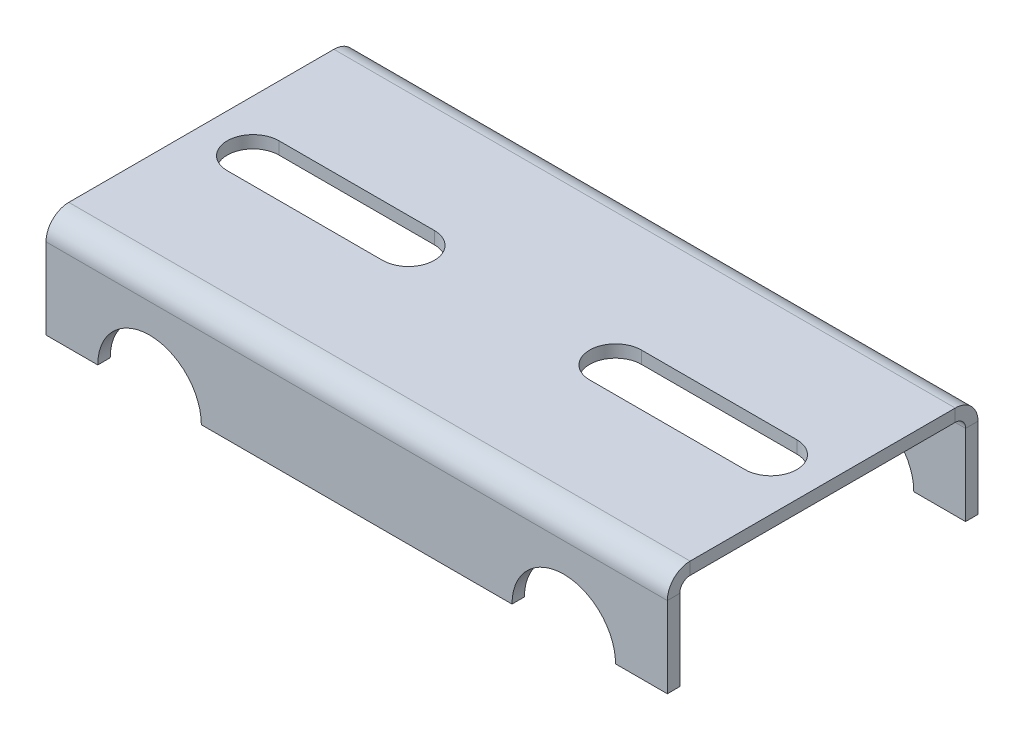
ISO-10303-21;
HEADER;
FILE_DESCRIPTION(('STEP AP214'),'2;1');
FILE_NAME('part.step','',(''),(''),'','','');
FILE_SCHEMA(('AUTOMOTIVE_DESIGN { 1 0 10303 214 1 1 1 1 }'));
ENDSEC;
DATA;
#1=APPLICATION_CONTEXT('core data for automotive mechanical design processes');
#2=APPLICATION_PROTOCOL_DEFINITION('international standard','automotive_design',2000,#1);
#3=PRODUCT_CONTEXT('',#1,'mechanical');
#4=PRODUCT('Part','Part','',(#3));
#5=PRODUCT_RELATED_PRODUCT_CATEGORY('part','',(#4));
#6=PRODUCT_DEFINITION_FORMATION('','',#4);
#7=PRODUCT_DEFINITION_CONTEXT('part definition',#1,'design');
#8=PRODUCT_DEFINITION('design','',#6,#7);
#9=PRODUCT_DEFINITION_SHAPE('','',#8);
#10=(LENGTH_UNIT() NAMED_UNIT(*) SI_UNIT(.MILLI.,.METRE.));
#11=(NAMED_UNIT(*) PLANE_ANGLE_UNIT() SI_UNIT($,.RADIAN.));
#12=(NAMED_UNIT(*) SI_UNIT($,.STERADIAN.) SOLID_ANGLE_UNIT());
#13=UNCERTAINTY_MEASURE_WITH_UNIT(LENGTH_MEASURE(1.E-05),#10,'distance_accuracy_value','');
#14=(GEOMETRIC_REPRESENTATION_CONTEXT(3) GLOBAL_UNCERTAINTY_ASSIGNED_CONTEXT((#13)) GLOBAL_UNIT_ASSIGNED_CONTEXT((#10,
#11,#12)) REPRESENTATION_CONTEXT('',''));
#15=CARTESIAN_POINT('',(0.,0.,0.));
#16=DIRECTION('',(0.,0.,1.));
#17=DIRECTION('',(1.,0.,0.));
#18=AXIS2_PLACEMENT_3D('',#15,#16,#17);
#19=CARTESIAN_POINT('',(0.,-1.524,0.));
#20=DIRECTION('',(0.,-1.,0.));
#21=DIRECTION('',(0.,0.,-1.));
#22=AXIS2_PLACEMENT_3D('',#19,#20,#21);
#23=PLANE('',#22);
#24=CARTESIAN_POINT('',(31.75,-1.524,0.));
#25=DIRECTION('',(0.,1.,0.));
#26=DIRECTION('',(0.,0.,-1.));
#27=AXIS2_PLACEMENT_3D('',#24,#25,#26);
#28=CIRCLE('',#27,3.175);
#29=CARTESIAN_POINT('',(31.75,-1.524,3.175));
#30=VERTEX_POINT('',#29);
#31=CARTESIAN_POINT('',(31.75,-1.524,-3.175));
#32=VERTEX_POINT('',#31);
#33=EDGE_CURVE('E476',#30,#32,#28,.T.);
#34=ORIENTED_EDGE('',*,*,#33,.T.);
#35=DIRECTION('',(-1.,0.,0.));
#36=VECTOR('',#35,1.);
#37=CARTESIAN_POINT('',(31.75,-1.524,-3.175));
#38=LINE('',#37,#36);
#39=CARTESIAN_POINT('',(12.7,-1.524,-3.175));
#40=VERTEX_POINT('',#39);
#41=EDGE_CURVE('E477',#32,#40,#38,.T.);
#42=ORIENTED_EDGE('',*,*,#41,.T.);
#43=CARTESIAN_POINT('',(12.7,-1.524,0.));
#44=DIRECTION('',(0.,1.,0.));
#45=DIRECTION('',(0.,0.,-1.));
#46=AXIS2_PLACEMENT_3D('',#43,#44,#45);
#47=CIRCLE('',#46,3.175);
#48=CARTESIAN_POINT('',(12.7,-1.524,3.175));
#49=VERTEX_POINT('',#48);
#50=EDGE_CURVE('E481',#40,#49,#47,.T.);
#51=ORIENTED_EDGE('',*,*,#50,.T.);
#52=DIRECTION('',(1.,0.,0.));
#53=VECTOR('',#52,1.);
#54=CARTESIAN_POINT('',(31.75,-1.524,3.175));
#55=LINE('',#54,#53);
#56=EDGE_CURVE('E488',#49,#30,#55,.T.);
#57=ORIENTED_EDGE('',*,*,#56,.T.);
#58=EDGE_LOOP('',(#34,#42,#51,#57));
#59=FACE_BOUND('',#58,.T.);
#60=CARTESIAN_POINT('',(-31.75,-1.524,0.));
#61=DIRECTION('',(0.,1.,0.));
#62=DIRECTION('',(0.,0.,1.));
#63=AXIS2_PLACEMENT_3D('',#60,#61,#62);
#64=CIRCLE('',#63,3.175);
#65=CARTESIAN_POINT('',(-31.75,-1.524,-3.175));
#66=VERTEX_POINT('',#65);
#67=CARTESIAN_POINT('',(-31.75,-1.524,3.175));
#68=VERTEX_POINT('',#67);
#69=EDGE_CURVE('E507',#66,#68,#64,.T.);
#70=ORIENTED_EDGE('',*,*,#69,.T.);
#71=DIRECTION('',(1.,0.,0.));
#72=VECTOR('',#71,1.);
#73=CARTESIAN_POINT('',(-31.75,-1.524,3.175));
#74=LINE('',#73,#72);
#75=CARTESIAN_POINT('',(-12.7,-1.524,3.175));
#76=VERTEX_POINT('',#75);
#77=EDGE_CURVE('E512',#68,#76,#74,.T.);
#78=ORIENTED_EDGE('',*,*,#77,.T.);
#79=CARTESIAN_POINT('',(-12.7,-1.524,0.));
#80=DIRECTION('',(0.,1.,0.));
#81=DIRECTION('',(0.,0.,1.));
#82=AXIS2_PLACEMENT_3D('',#79,#80,#81);
#83=CIRCLE('',#82,3.175);
#84=CARTESIAN_POINT('',(-12.7,-1.524,-3.175));
#85=VERTEX_POINT('',#84);
#86=EDGE_CURVE('E513',#76,#85,#83,.T.);
#87=ORIENTED_EDGE('',*,*,#86,.T.);
#88=DIRECTION('',(-1.,0.,0.));
#89=VECTOR('',#88,1.);
#90=CARTESIAN_POINT('',(-31.75,-1.524,-3.175));
#91=LINE('',#90,#89);
#92=EDGE_CURVE('E520',#85,#66,#91,.T.);
#93=ORIENTED_EDGE('',*,*,#92,.T.);
#94=EDGE_LOOP('',(#70,#78,#87,#93));
#95=FACE_BOUND('',#94,.T.);
#96=DIRECTION('',(0.,0.,1.));
#97=VECTOR('',#96,1.);
#98=CARTESIAN_POINT('',(-38.1,-1.524,19.05));
#99=LINE('',#98,#97);
#100=CARTESIAN_POINT('',(-38.1,-1.52400000000001,-16.256));
#101=VERTEX_POINT('',#100);
#102=CARTESIAN_POINT('',(-38.1,-1.524,16.256));
#103=VERTEX_POINT('',#102);
#104=EDGE_CURVE('E13',#101,#103,#99,.T.);
#105=ORIENTED_EDGE('',*,*,#104,.F.);
#106=DIRECTION('',(1.,0.,0.));
#107=VECTOR('',#106,1.);
#108=CARTESIAN_POINT('',(38.1,-1.52400000000001,-16.256));
#109=LINE('',#108,#107);
#110=CARTESIAN_POINT('',(38.1,-1.52400000000001,-16.256));
#111=VERTEX_POINT('',#110);
#112=EDGE_CURVE('E385',#111,#101,#109,.F.);
#113=ORIENTED_EDGE('',*,*,#112,.F.);
#114=DIRECTION('',(0.,0.,-1.));
#115=VECTOR('',#114,1.);
#116=CARTESIAN_POINT('',(38.1,-1.524,19.05));
#117=LINE('',#116,#115);
#118=CARTESIAN_POINT('',(38.1,-1.524,16.256));
#119=VERTEX_POINT('',#118);
#120=EDGE_CURVE('E127',#119,#111,#117,.T.);
#121=ORIENTED_EDGE('',*,*,#120,.F.);
#122=DIRECTION('',(-1.,0.,0.));
#123=VECTOR('',#122,1.);
#124=CARTESIAN_POINT('',(-38.1,-1.524,16.256));
#125=LINE('',#124,#123);
#126=EDGE_CURVE('E466',#103,#119,#125,.F.);
#127=ORIENTED_EDGE('',*,*,#126,.F.);
#128=EDGE_LOOP('',(#105,#113,#121,#127));
#129=FACE_BOUND('',#128,.T.);
#130=ADVANCED_FACE('F122',(#59,#95,#129),#23,.T.);
#131=CARTESIAN_POINT('',(0.,0.,0.));
#132=DIRECTION('',(0.,-1.,0.));
#133=DIRECTION('',(0.,0.,-1.));
#134=AXIS2_PLACEMENT_3D('',#131,#132,#133);
#135=PLANE('',#134);
#136=DIRECTION('',(-1.,0.,0.));
#137=VECTOR('',#136,1.);
#138=CARTESIAN_POINT('',(31.75,0.,-3.175));
#139=LINE('',#138,#137);
#140=CARTESIAN_POINT('',(31.75,0.,-3.175));
#141=VERTEX_POINT('',#140);
#142=CARTESIAN_POINT('',(12.7,0.,-3.175));
#143=VERTEX_POINT('',#142);
#144=EDGE_CURVE('E493',#141,#143,#139,.T.);
#145=ORIENTED_EDGE('',*,*,#144,.F.);
#146=CARTESIAN_POINT('',(31.75,0.,0.));
#147=DIRECTION('',(0.,1.,0.));
#148=DIRECTION('',(0.,0.,-1.));
#149=AXIS2_PLACEMENT_3D('',#146,#147,#148);
#150=CIRCLE('',#149,3.175);
#151=CARTESIAN_POINT('',(31.75,0.,3.175));
#152=VERTEX_POINT('',#151);
#153=EDGE_CURVE('E473',#152,#141,#150,.T.);
#154=ORIENTED_EDGE('',*,*,#153,.F.);
#155=DIRECTION('',(1.,0.,0.));
#156=VECTOR('',#155,1.);
#157=CARTESIAN_POINT('',(31.75,0.,3.175));
#158=LINE('',#157,#156);
#159=CARTESIAN_POINT('',(12.7,0.,3.175));
#160=VERTEX_POINT('',#159);
#161=EDGE_CURVE('E479',#160,#152,#158,.T.);
#162=ORIENTED_EDGE('',*,*,#161,.F.);
#163=CARTESIAN_POINT('',(12.7,0.,0.));
#164=DIRECTION('',(0.,1.,0.));
#165=DIRECTION('',(0.,0.,-1.));
#166=AXIS2_PLACEMENT_3D('',#163,#164,#165);
#167=CIRCLE('',#166,3.175);
#168=EDGE_CURVE('E494',#143,#160,#167,.T.);
#169=ORIENTED_EDGE('',*,*,#168,.F.);
#170=EDGE_LOOP('',(#145,#154,#162,#169));
#171=FACE_BOUND('',#170,.T.);
#172=DIRECTION('',(1.,0.,0.));
#173=VECTOR('',#172,1.);
#174=CARTESIAN_POINT('',(-31.75,0.,3.175));
#175=LINE('',#174,#173);
#176=CARTESIAN_POINT('',(-31.75,0.,3.175));
#177=VERTEX_POINT('',#176);
#178=CARTESIAN_POINT('',(-12.7,0.,3.175));
#179=VERTEX_POINT('',#178);
#180=EDGE_CURVE('E525',#177,#179,#175,.T.);
#181=ORIENTED_EDGE('',*,*,#180,.F.);
#182=CARTESIAN_POINT('',(-31.75,0.,0.));
#183=DIRECTION('',(0.,1.,0.));
#184=DIRECTION('',(0.,0.,1.));
#185=AXIS2_PLACEMENT_3D('',#182,#183,#184);
#186=CIRCLE('',#185,3.175);
#187=CARTESIAN_POINT('',(-31.75,0.,-3.175));
#188=VERTEX_POINT('',#187);
#189=EDGE_CURVE('E501',#188,#177,#186,.T.);
#190=ORIENTED_EDGE('',*,*,#189,.F.);
#191=DIRECTION('',(-1.,0.,0.));
#192=VECTOR('',#191,1.);
#193=CARTESIAN_POINT('',(-31.75,0.,-3.175));
#194=LINE('',#193,#192);
#195=CARTESIAN_POINT('',(-12.7,0.,-3.175));
#196=VERTEX_POINT('',#195);
#197=EDGE_CURVE('E515',#196,#188,#194,.T.);
#198=ORIENTED_EDGE('',*,*,#197,.F.);
#199=CARTESIAN_POINT('',(-12.7,0.,0.));
#200=DIRECTION('',(0.,1.,0.));
#201=DIRECTION('',(0.,0.,1.));
#202=AXIS2_PLACEMENT_3D('',#199,#200,#201);
#203=CIRCLE('',#202,3.175);
#204=EDGE_CURVE('E528',#179,#196,#203,.T.);
#205=ORIENTED_EDGE('',*,*,#204,.F.);
#206=EDGE_LOOP('',(#181,#190,#198,#205));
#207=FACE_BOUND('',#206,.T.);
#208=DIRECTION('',(1.,0.,0.));
#209=VECTOR('',#208,1.);
#210=CARTESIAN_POINT('',(38.1,0.,-16.256));
#211=LINE('',#210,#209);
#212=CARTESIAN_POINT('',(38.1,0.,-16.256));
#213=VERTEX_POINT('',#212);
#214=CARTESIAN_POINT('',(-38.1,0.,-16.256));
#215=VERTEX_POINT('',#214);
#216=EDGE_CURVE('E369',#213,#215,#211,.F.);
#217=ORIENTED_EDGE('',*,*,#216,.T.);
#218=DIRECTION('',(0.,0.,1.));
#219=VECTOR('',#218,1.);
#220=CARTESIAN_POINT('',(-38.1,0.,19.05));
#221=LINE('',#220,#219);
#222=CARTESIAN_POINT('',(-38.1,0.,16.256));
#223=VERTEX_POINT('',#222);
#224=EDGE_CURVE('E123',#215,#223,#221,.T.);
#225=ORIENTED_EDGE('',*,*,#224,.T.);
#226=DIRECTION('',(-1.,0.,0.));
#227=VECTOR('',#226,1.);
#228=CARTESIAN_POINT('',(-38.1,0.,16.256));
#229=LINE('',#228,#227);
#230=CARTESIAN_POINT('',(38.1,0.,16.256));
#231=VERTEX_POINT('',#230);
#232=EDGE_CURVE('E459',#223,#231,#229,.F.);
#233=ORIENTED_EDGE('',*,*,#232,.T.);
#234=DIRECTION('',(0.,0.,-1.));
#235=VECTOR('',#234,1.);
#236=CARTESIAN_POINT('',(38.1,0.,19.05));
#237=LINE('',#236,#235);
#238=EDGE_CURVE('E531',#231,#213,#237,.T.);
#239=ORIENTED_EDGE('',*,*,#238,.T.);
#240=EDGE_LOOP('',(#217,#225,#233,#239));
#241=FACE_BOUND('',#240,.T.);
#242=ADVANCED_FACE('F545',(#171,#207,#241),#135,.F.);
#243=CARTESIAN_POINT('',(38.1,-1.524,19.05));
#244=DIRECTION('',(1.,0.,0.));
#245=DIRECTION('',(0.,0.,-1.));
#246=AXIS2_PLACEMENT_3D('',#243,#244,#245);
#247=PLANE('',#246);
#248=ORIENTED_EDGE('',*,*,#120,.T.);
#249=DIRECTION('',(0.,1.,0.));
#250=VECTOR('',#249,1.);
#251=CARTESIAN_POINT('',(38.1,-1.52400000000001,-16.256));
#252=LINE('',#251,#250);
#253=EDGE_CURVE('E376',#111,#213,#252,.T.);
#254=ORIENTED_EDGE('',*,*,#253,.T.);
#255=ORIENTED_EDGE('',*,*,#238,.F.);
#256=DIRECTION('',(0.,1.,0.));
#257=VECTOR('',#256,1.);
#258=CARTESIAN_POINT('',(38.1,-1.524,16.256));
#259=LINE('',#258,#257);
#260=EDGE_CURVE('E144',#119,#231,#259,.T.);
#261=ORIENTED_EDGE('',*,*,#260,.F.);
#262=EDGE_LOOP('',(#248,#254,#255,#261));
#263=FACE_BOUND('',#262,.T.);
#264=ADVANCED_FACE('F124',(#263),#247,.T.);
#265=CARTESIAN_POINT('',(-38.1,-1.524,19.05));
#266=DIRECTION('',(-1.,0.,0.));
#267=DIRECTION('',(0.,0.,1.));
#268=AXIS2_PLACEMENT_3D('',#265,#266,#267);
#269=PLANE('',#268);
#270=DIRECTION('',(0.,1.,0.));
#271=VECTOR('',#270,1.);
#272=CARTESIAN_POINT('',(-38.1,-1.52400000000001,-16.256));
#273=LINE('',#272,#271);
#274=EDGE_CURVE('E386',#101,#215,#273,.T.);
#275=ORIENTED_EDGE('',*,*,#274,.F.);
#276=ORIENTED_EDGE('',*,*,#104,.T.);
#277=DIRECTION('',(0.,1.,0.));
#278=VECTOR('',#277,1.);
#279=CARTESIAN_POINT('',(-38.1,-1.524,16.256));
#280=LINE('',#279,#278);
#281=EDGE_CURVE('E464',#103,#223,#280,.T.);
#282=ORIENTED_EDGE('',*,*,#281,.T.);
#283=ORIENTED_EDGE('',*,*,#224,.F.);
#284=EDGE_LOOP('',(#275,#276,#282,#283));
#285=FACE_BOUND('',#284,.T.);
#286=ADVANCED_FACE('F548',(#285),#269,.T.);
#287=CARTESIAN_POINT('',(-31.75,-1.524,0.));
#288=DIRECTION('',(0.,1.,0.));
#289=DIRECTION('',(0.,0.,1.));
#290=AXIS2_PLACEMENT_3D('',#287,#288,#289);
#291=CYLINDRICAL_SURFACE('',#290,3.175);
#292=ORIENTED_EDGE('',*,*,#189,.T.);
#293=DIRECTION('',(0.,1.,0.));
#294=VECTOR('',#293,1.);
#295=CARTESIAN_POINT('',(-31.75,-1.524,3.175));
#296=LINE('',#295,#294);
#297=EDGE_CURVE('E524',#68,#177,#296,.T.);
#298=ORIENTED_EDGE('',*,*,#297,.F.);
#299=ORIENTED_EDGE('',*,*,#69,.F.);
#300=DIRECTION('',(0.,1.,0.));
#301=VECTOR('',#300,1.);
#302=CARTESIAN_POINT('',(-31.75,-1.524,-3.175));
#303=LINE('',#302,#301);
#304=EDGE_CURVE('E532',#66,#188,#303,.T.);
#305=ORIENTED_EDGE('',*,*,#304,.T.);
#306=EDGE_LOOP('',(#292,#298,#299,#305));
#307=FACE_BOUND('',#306,.T.);
#308=ADVANCED_FACE('F612',(#307),#291,.F.);
#309=CARTESIAN_POINT('',(-31.75,-1.524,-3.175));
#310=DIRECTION('',(0.,0.,-1.));
#311=DIRECTION('',(-1.,0.,0.));
#312=AXIS2_PLACEMENT_3D('',#309,#310,#311);
#313=PLANE('',#312);
#314=ORIENTED_EDGE('',*,*,#197,.T.);
#315=ORIENTED_EDGE('',*,*,#304,.F.);
#316=ORIENTED_EDGE('',*,*,#92,.F.);
#317=DIRECTION('',(0.,1.,0.));
#318=VECTOR('',#317,1.);
#319=CARTESIAN_POINT('',(-12.7,-1.524,-3.175));
#320=LINE('',#319,#318);
#321=EDGE_CURVE('E534',#85,#196,#320,.T.);
#322=ORIENTED_EDGE('',*,*,#321,.T.);
#323=EDGE_LOOP('',(#314,#315,#316,#322));
#324=FACE_BOUND('',#323,.T.);
#325=ADVANCED_FACE('F625',(#324),#313,.F.);
#326=CARTESIAN_POINT('',(-12.7,-1.524,0.));
#327=DIRECTION('',(0.,1.,0.));
#328=DIRECTION('',(0.,0.,1.));
#329=AXIS2_PLACEMENT_3D('',#326,#327,#328);
#330=CYLINDRICAL_SURFACE('',#329,3.175);
#331=ORIENTED_EDGE('',*,*,#204,.T.);
#332=ORIENTED_EDGE('',*,*,#321,.F.);
#333=ORIENTED_EDGE('',*,*,#86,.F.);
#334=DIRECTION('',(0.,1.,0.));
#335=VECTOR('',#334,1.);
#336=CARTESIAN_POINT('',(-12.7,-1.524,3.175));
#337=LINE('',#336,#335);
#338=EDGE_CURVE('E539',#76,#179,#337,.T.);
#339=ORIENTED_EDGE('',*,*,#338,.T.);
#340=EDGE_LOOP('',(#331,#332,#333,#339));
#341=FACE_BOUND('',#340,.T.);
#342=ADVANCED_FACE('F941',(#341),#330,.F.);
#343=CARTESIAN_POINT('',(-31.75,-1.524,3.175));
#344=DIRECTION('',(0.,0.,1.));
#345=DIRECTION('',(1.,0.,0.));
#346=AXIS2_PLACEMENT_3D('',#343,#344,#345);
#347=PLANE('',#346);
#348=ORIENTED_EDGE('',*,*,#180,.T.);
#349=ORIENTED_EDGE('',*,*,#338,.F.);
#350=ORIENTED_EDGE('',*,*,#77,.F.);
#351=ORIENTED_EDGE('',*,*,#297,.T.);
#352=EDGE_LOOP('',(#348,#349,#350,#351));
#353=FACE_BOUND('',#352,.T.);
#354=ADVANCED_FACE('F932',(#353),#347,.F.);
#355=CARTESIAN_POINT('',(31.75,-1.524,0.));
#356=DIRECTION('',(0.,1.,0.));
#357=DIRECTION('',(0.,0.,1.));
#358=AXIS2_PLACEMENT_3D('',#355,#356,#357);
#359=CYLINDRICAL_SURFACE('',#358,3.175);
#360=ORIENTED_EDGE('',*,*,#153,.T.);
#361=DIRECTION('',(0.,1.,0.));
#362=VECTOR('',#361,1.);
#363=CARTESIAN_POINT('',(31.75,-1.524,-3.175));
#364=LINE('',#363,#362);
#365=EDGE_CURVE('E490',#32,#141,#364,.T.);
#366=ORIENTED_EDGE('',*,*,#365,.F.);
#367=ORIENTED_EDGE('',*,*,#33,.F.);
#368=DIRECTION('',(0.,1.,0.));
#369=VECTOR('',#368,1.);
#370=CARTESIAN_POINT('',(31.75,-1.524,3.175));
#371=LINE('',#370,#369);
#372=EDGE_CURVE('E497',#30,#152,#371,.T.);
#373=ORIENTED_EDGE('',*,*,#372,.T.);
#374=EDGE_LOOP('',(#360,#366,#367,#373));
#375=FACE_BOUND('',#374,.T.);
#376=ADVANCED_FACE('F923',(#375),#359,.F.);
#377=CARTESIAN_POINT('',(31.75,-1.524,3.175));
#378=DIRECTION('',(0.,0.,1.));
#379=DIRECTION('',(1.,0.,0.));
#380=AXIS2_PLACEMENT_3D('',#377,#378,#379);
#381=PLANE('',#380);
#382=ORIENTED_EDGE('',*,*,#161,.T.);
#383=ORIENTED_EDGE('',*,*,#372,.F.);
#384=ORIENTED_EDGE('',*,*,#56,.F.);
#385=DIRECTION('',(0.,1.,0.));
#386=VECTOR('',#385,1.);
#387=CARTESIAN_POINT('',(12.7,-1.524,3.175));
#388=LINE('',#387,#386);
#389=EDGE_CURVE('E505',#49,#160,#388,.T.);
#390=ORIENTED_EDGE('',*,*,#389,.T.);
#391=EDGE_LOOP('',(#382,#383,#384,#390));
#392=FACE_BOUND('',#391,.T.);
#393=ADVANCED_FACE('F918',(#392),#381,.F.);
#394=CARTESIAN_POINT('',(12.7,-1.524,0.));
#395=DIRECTION('',(0.,1.,0.));
#396=DIRECTION('',(0.,0.,1.));
#397=AXIS2_PLACEMENT_3D('',#394,#395,#396);
#398=CYLINDRICAL_SURFACE('',#397,3.175);
#399=ORIENTED_EDGE('',*,*,#168,.T.);
#400=ORIENTED_EDGE('',*,*,#389,.F.);
#401=ORIENTED_EDGE('',*,*,#50,.F.);
#402=DIRECTION('',(0.,1.,0.));
#403=VECTOR('',#402,1.);
#404=CARTESIAN_POINT('',(12.7,-1.524,-3.175));
#405=LINE('',#404,#403);
#406=EDGE_CURVE('E502',#40,#143,#405,.T.);
#407=ORIENTED_EDGE('',*,*,#406,.T.);
#408=EDGE_LOOP('',(#399,#400,#401,#407));
#409=FACE_BOUND('',#408,.T.);
#410=ADVANCED_FACE('F906',(#409),#398,.F.);
#411=CARTESIAN_POINT('',(31.75,-1.524,-3.175));
#412=DIRECTION('',(0.,0.,-1.));
#413=DIRECTION('',(-1.,0.,0.));
#414=AXIS2_PLACEMENT_3D('',#411,#412,#413);
#415=PLANE('',#414);
#416=ORIENTED_EDGE('',*,*,#144,.T.);
#417=ORIENTED_EDGE('',*,*,#406,.F.);
#418=ORIENTED_EDGE('',*,*,#41,.F.);
#419=ORIENTED_EDGE('',*,*,#365,.T.);
#420=EDGE_LOOP('',(#416,#417,#418,#419));
#421=FACE_BOUND('',#420,.T.);
#422=ADVANCED_FACE('F892',(#421),#415,.F.);
#423=CARTESIAN_POINT('',(38.1,-2.794,16.256));
#424=DIRECTION('',(1.,0.,0.));
#425=DIRECTION('',(0.,0.,-1.));
#426=AXIS2_PLACEMENT_3D('',#423,#424,#425);
#427=PLANE('',#426);
#428=DIRECTION('',(0.,0.,1.));
#429=VECTOR('',#428,1.);
#430=CARTESIAN_POINT('',(38.1,-2.794,19.05));
#431=LINE('',#430,#429);
#432=CARTESIAN_POINT('',(38.1,-2.79399999999999,17.526));
#433=VERTEX_POINT('',#432);
#434=CARTESIAN_POINT('',(38.1,-2.79399999999999,19.05));
#435=VERTEX_POINT('',#434);
#436=EDGE_CURVE('E387',#433,#435,#431,.T.);
#437=ORIENTED_EDGE('',*,*,#436,.F.);
#438=CARTESIAN_POINT('',(38.1,-2.794,16.256));
#439=DIRECTION('',(-1.,0.,0.));
#440=DIRECTION('',(0.,0.,1.));
#441=AXIS2_PLACEMENT_3D('',#438,#439,#440);
#442=CIRCLE('',#441,1.27);
#443=EDGE_CURVE('E461',#119,#433,#442,.F.);
#444=ORIENTED_EDGE('',*,*,#443,.F.);
#445=ORIENTED_EDGE('',*,*,#260,.T.);
#446=CARTESIAN_POINT('',(38.1,-2.794,16.256));
#447=DIRECTION('',(-1.,0.,0.));
#448=DIRECTION('',(0.,0.,1.));
#449=AXIS2_PLACEMENT_3D('',#446,#447,#448);
#450=CIRCLE('',#449,2.794);
#451=EDGE_CURVE('E460',#231,#435,#450,.F.);
#452=ORIENTED_EDGE('',*,*,#451,.T.);
#453=EDGE_LOOP('',(#437,#444,#445,#452));
#454=FACE_BOUND('',#453,.T.);
#455=ADVANCED_FACE('F590',(#454),#427,.T.);
#456=CARTESIAN_POINT('',(-38.1,-2.794,16.256));
#457=DIRECTION('',(1.,0.,0.));
#458=DIRECTION('',(0.,0.,-1.));
#459=AXIS2_PLACEMENT_3D('',#456,#457,#458);
#460=PLANE('',#459);
#461=CARTESIAN_POINT('',(-38.1,-2.794,16.256));
#462=DIRECTION('',(-1.,0.,0.));
#463=DIRECTION('',(0.,0.,1.));
#464=AXIS2_PLACEMENT_3D('',#461,#462,#463);
#465=CIRCLE('',#464,1.27);
#466=CARTESIAN_POINT('',(-38.1,-2.79399999999999,17.526));
#467=VERTEX_POINT('',#466);
#468=EDGE_CURVE('E392',#467,#103,#465,.T.);
#469=ORIENTED_EDGE('',*,*,#468,.F.);
#470=DIRECTION('',(0.,0.,1.));
#471=VECTOR('',#470,1.);
#472=CARTESIAN_POINT('',(-38.1,-2.794,17.526));
#473=LINE('',#472,#471);
#474=CARTESIAN_POINT('',(-38.1,-2.794,19.05));
#475=VERTEX_POINT('',#474);
#476=EDGE_CURVE('E446',#467,#475,#473,.T.);
#477=ORIENTED_EDGE('',*,*,#476,.T.);
#478=CARTESIAN_POINT('',(-38.1,-2.794,16.256));
#479=DIRECTION('',(-1.,0.,0.));
#480=DIRECTION('',(0.,0.,1.));
#481=AXIS2_PLACEMENT_3D('',#478,#479,#480);
#482=CIRCLE('',#481,2.794);
#483=EDGE_CURVE('E458',#475,#223,#482,.T.);
#484=ORIENTED_EDGE('',*,*,#483,.T.);
#485=ORIENTED_EDGE('',*,*,#281,.F.);
#486=EDGE_LOOP('',(#469,#477,#484,#485));
#487=FACE_BOUND('',#486,.T.);
#488=ADVANCED_FACE('F552',(#487),#460,.F.);
#489=CARTESIAN_POINT('',(-38.1,-2.794,16.256));
#490=DIRECTION('',(-1.,0.,0.));
#491=DIRECTION('',(0.,0.,1.));
#492=AXIS2_PLACEMENT_3D('',#489,#490,#491);
#493=CYLINDRICAL_SURFACE('',#492,2.794);
#494=ORIENTED_EDGE('',*,*,#232,.F.);
#495=ORIENTED_EDGE('',*,*,#483,.F.);
#496=DIRECTION('',(-1.,0.,0.));
#497=VECTOR('',#496,1.);
#498=CARTESIAN_POINT('',(38.1,-2.794,19.05));
#499=LINE('',#498,#497);
#500=EDGE_CURVE('E450',#475,#435,#499,.F.);
#501=ORIENTED_EDGE('',*,*,#500,.T.);
#502=ORIENTED_EDGE('',*,*,#451,.F.);
#503=EDGE_LOOP('',(#494,#495,#501,#502));
#504=FACE_BOUND('',#503,.T.);
#505=ADVANCED_FACE('F553',(#504),#493,.T.);
#506=CARTESIAN_POINT('',(-38.1,-2.794,16.256));
#507=DIRECTION('',(-1.,0.,0.));
#508=DIRECTION('',(0.,0.,1.));
#509=AXIS2_PLACEMENT_3D('',#506,#507,#508);
#510=CYLINDRICAL_SURFACE('',#509,1.27);
#511=ORIENTED_EDGE('',*,*,#126,.T.);
#512=ORIENTED_EDGE('',*,*,#443,.T.);
#513=DIRECTION('',(-1.,0.,0.));
#514=VECTOR('',#513,1.);
#515=CARTESIAN_POINT('',(38.1,-2.794,17.526));
#516=LINE('',#515,#514);
#517=EDGE_CURVE('E451',#433,#467,#516,.T.);
#518=ORIENTED_EDGE('',*,*,#517,.T.);
#519=ORIENTED_EDGE('',*,*,#468,.T.);
#520=EDGE_LOOP('',(#511,#512,#518,#519));
#521=FACE_BOUND('',#520,.T.);
#522=ADVANCED_FACE('F593',(#521),#510,.F.);
#523=CARTESIAN_POINT('',(-38.1,-1.52399999999999,19.05));
#524=DIRECTION('',(-1.,0.,0.));
#525=DIRECTION('',(0.,-1.,0.));
#526=AXIS2_PLACEMENT_3D('',#523,#524,#525);
#527=PLANE('',#526);
#528=DIRECTION('',(0.,-1.,0.));
#529=VECTOR('',#528,1.);
#530=CARTESIAN_POINT('',(-38.1,-1.52399999999999,19.05));
#531=LINE('',#530,#529);
#532=CARTESIAN_POINT('',(-38.1,-12.7,19.05));
#533=VERTEX_POINT('',#532);
#534=EDGE_CURVE('E406',#533,#475,#531,.F.);
#535=ORIENTED_EDGE('',*,*,#534,.T.);
#536=ORIENTED_EDGE('',*,*,#476,.F.);
#537=DIRECTION('',(0.,1.,0.));
#538=VECTOR('',#537,1.);
#539=CARTESIAN_POINT('',(-38.1,-12.7,17.526));
#540=LINE('',#539,#538);
#541=CARTESIAN_POINT('',(-38.1,-12.7,17.526));
#542=VERTEX_POINT('',#541);
#543=EDGE_CURVE('E430',#542,#467,#540,.T.);
#544=ORIENTED_EDGE('',*,*,#543,.F.);
#545=DIRECTION('',(0.,0.,-1.));
#546=VECTOR('',#545,1.);
#547=CARTESIAN_POINT('',(-38.1,-12.7,19.05));
#548=LINE('',#547,#546);
#549=EDGE_CURVE('E395',#533,#542,#548,.T.);
#550=ORIENTED_EDGE('',*,*,#549,.F.);
#551=EDGE_LOOP('',(#535,#536,#544,#550));
#552=FACE_BOUND('',#551,.T.);
#553=ADVANCED_FACE('F563',(#552),#527,.T.);
#554=CARTESIAN_POINT('',(38.1,-12.7,19.05));
#555=DIRECTION('',(1.,0.,0.));
#556=DIRECTION('',(0.,1.,0.));
#557=AXIS2_PLACEMENT_3D('',#554,#555,#556);
#558=PLANE('',#557);
#559=DIRECTION('',(0.,-1.,0.));
#560=VECTOR('',#559,1.);
#561=CARTESIAN_POINT('',(38.1,-12.6999999999999,17.526));
#562=LINE('',#561,#560);
#563=CARTESIAN_POINT('',(38.1,-12.6999999999998,17.526));
#564=VERTEX_POINT('',#563);
#565=EDGE_CURVE('E444',#433,#564,#562,.T.);
#566=ORIENTED_EDGE('',*,*,#565,.F.);
#567=ORIENTED_EDGE('',*,*,#436,.T.);
#568=DIRECTION('',(0.,1.,0.));
#569=VECTOR('',#568,1.);
#570=CARTESIAN_POINT('',(38.1,-12.7,19.05));
#571=LINE('',#570,#569);
#572=CARTESIAN_POINT('',(38.1,-12.7,19.05));
#573=VERTEX_POINT('',#572);
#574=EDGE_CURVE('E424',#435,#573,#571,.F.);
#575=ORIENTED_EDGE('',*,*,#574,.T.);
#576=DIRECTION('',(0.,0.,-1.));
#577=VECTOR('',#576,1.);
#578=CARTESIAN_POINT('',(38.1,-12.7,19.05));
#579=LINE('',#578,#577);
#580=EDGE_CURVE('E404',#573,#564,#579,.T.);
#581=ORIENTED_EDGE('',*,*,#580,.T.);
#582=EDGE_LOOP('',(#566,#567,#575,#581));
#583=FACE_BOUND('',#582,.T.);
#584=ADVANCED_FACE('F582',(#583),#558,.T.);
#585=CARTESIAN_POINT('',(-25.4,-12.7,19.05));
#586=DIRECTION('',(0.,0.,-1.));
#587=DIRECTION('',(0.,1.,0.));
#588=AXIS2_PLACEMENT_3D('',#585,#586,#587);
#589=PLANE('',#588);
#590=ORIENTED_EDGE('',*,*,#500,.F.);
#591=ORIENTED_EDGE('',*,*,#534,.F.);
#592=DIRECTION('',(1.,0.,0.));
#593=VECTOR('',#592,1.);
#594=CARTESIAN_POINT('',(-38.1,-12.7,19.05));
#595=LINE('',#594,#593);
#596=CARTESIAN_POINT('',(-31.75,-12.7,19.05));
#597=VERTEX_POINT('',#596);
#598=EDGE_CURVE('E407',#597,#533,#595,.F.);
#599=ORIENTED_EDGE('',*,*,#598,.F.);
#600=CARTESIAN_POINT('',(-25.4,-12.7,19.05));
#601=DIRECTION('',(0.,0.,-1.));
#602=DIRECTION('',(0.,1.,0.));
#603=AXIS2_PLACEMENT_3D('',#600,#601,#602);
#604=CIRCLE('',#603,6.35);
#605=CARTESIAN_POINT('',(-19.05,-12.7,19.05));
#606=VERTEX_POINT('',#605);
#607=EDGE_CURVE('E413',#606,#597,#604,.F.);
#608=ORIENTED_EDGE('',*,*,#607,.F.);
#609=DIRECTION('',(1.,0.,0.));
#610=VECTOR('',#609,1.);
#611=CARTESIAN_POINT('',(-19.05,-12.7,19.05));
#612=LINE('',#611,#610);
#613=CARTESIAN_POINT('',(19.05,-12.7,19.05));
#614=VERTEX_POINT('',#613);
#615=EDGE_CURVE('E418',#614,#606,#612,.F.);
#616=ORIENTED_EDGE('',*,*,#615,.F.);
#617=CARTESIAN_POINT('',(25.4,-12.7,19.05));
#618=DIRECTION('',(0.,0.,-1.));
#619=DIRECTION('',(0.,1.,0.));
#620=AXIS2_PLACEMENT_3D('',#617,#618,#619);
#621=CIRCLE('',#620,6.35);
#622=CARTESIAN_POINT('',(31.75,-12.7,19.05));
#623=VERTEX_POINT('',#622);
#624=EDGE_CURVE('E417',#623,#614,#621,.F.);
#625=ORIENTED_EDGE('',*,*,#624,.F.);
#626=DIRECTION('',(1.,0.,0.));
#627=VECTOR('',#626,1.);
#628=CARTESIAN_POINT('',(31.75,-12.7,19.05));
#629=LINE('',#628,#627);
#630=EDGE_CURVE('E422',#573,#623,#629,.F.);
#631=ORIENTED_EDGE('',*,*,#630,.F.);
#632=ORIENTED_EDGE('',*,*,#574,.F.);
#633=EDGE_LOOP('',(#590,#591,#599,#608,#616,#625,#631,#632));
#634=FACE_BOUND('',#633,.T.);
#635=ADVANCED_FACE('F557',(#634),#589,.F.);
#636=CARTESIAN_POINT('',(-25.4,-12.7,17.526));
#637=DIRECTION('',(0.,0.,-1.));
#638=DIRECTION('',(0.,1.,0.));
#639=AXIS2_PLACEMENT_3D('',#636,#637,#638);
#640=PLANE('',#639);
#641=ORIENTED_EDGE('',*,*,#543,.T.);
#642=ORIENTED_EDGE('',*,*,#517,.F.);
#643=ORIENTED_EDGE('',*,*,#565,.T.);
#644=DIRECTION('',(-1.,0.,0.));
#645=VECTOR('',#644,1.);
#646=CARTESIAN_POINT('',(-25.4,-12.7,17.526));
#647=LINE('',#646,#645);
#648=CARTESIAN_POINT('',(31.75,-12.6999999999998,17.526));
#649=VERTEX_POINT('',#648);
#650=EDGE_CURVE('E445',#564,#649,#647,.T.);
#651=ORIENTED_EDGE('',*,*,#650,.T.);
#652=CARTESIAN_POINT('',(25.4,-12.7,17.526));
#653=DIRECTION('',(0.,0.,-1.));
#654=DIRECTION('',(0.,1.,0.));
#655=AXIS2_PLACEMENT_3D('',#652,#653,#654);
#656=CIRCLE('',#655,6.35);
#657=CARTESIAN_POINT('',(19.05,-12.7,17.526));
#658=VERTEX_POINT('',#657);
#659=EDGE_CURVE('E437',#649,#658,#656,.F.);
#660=ORIENTED_EDGE('',*,*,#659,.T.);
#661=DIRECTION('',(-1.,0.,0.));
#662=VECTOR('',#661,1.);
#663=CARTESIAN_POINT('',(-25.4,-12.7,17.526));
#664=LINE('',#663,#662);
#665=CARTESIAN_POINT('',(-19.05,-12.7,17.526));
#666=VERTEX_POINT('',#665);
#667=EDGE_CURVE('E436',#658,#666,#664,.T.);
#668=ORIENTED_EDGE('',*,*,#667,.T.);
#669=CARTESIAN_POINT('',(-25.4,-12.7,17.526));
#670=DIRECTION('',(0.,0.,-1.));
#671=DIRECTION('',(0.,1.,0.));
#672=AXIS2_PLACEMENT_3D('',#669,#670,#671);
#673=CIRCLE('',#672,6.35);
#674=CARTESIAN_POINT('',(-31.75,-12.7,17.526));
#675=VERTEX_POINT('',#674);
#676=EDGE_CURVE('E433',#666,#675,#673,.F.);
#677=ORIENTED_EDGE('',*,*,#676,.T.);
#678=DIRECTION('',(-1.,0.,0.));
#679=VECTOR('',#678,1.);
#680=CARTESIAN_POINT('',(-25.4,-12.7,17.526));
#681=LINE('',#680,#679);
#682=EDGE_CURVE('E427',#675,#542,#681,.T.);
#683=ORIENTED_EDGE('',*,*,#682,.T.);
#684=EDGE_LOOP('',(#641,#642,#643,#651,#660,#668,#677,#683));
#685=FACE_BOUND('',#684,.T.);
#686=ADVANCED_FACE('F592',(#685),#640,.T.);
#687=CARTESIAN_POINT('',(-38.1,-12.7,19.05));
#688=DIRECTION('',(0.,-1.,0.));
#689=DIRECTION('',(0.,0.,-1.));
#690=AXIS2_PLACEMENT_3D('',#687,#688,#689);
#691=PLANE('',#690);
#692=ORIENTED_EDGE('',*,*,#682,.F.);
#693=DIRECTION('',(0.,0.,-1.));
#694=VECTOR('',#693,1.);
#695=CARTESIAN_POINT('',(-31.75,-12.7,19.05));
#696=LINE('',#695,#694);
#697=EDGE_CURVE('E398',#597,#675,#696,.T.);
#698=ORIENTED_EDGE('',*,*,#697,.F.);
#699=ORIENTED_EDGE('',*,*,#598,.T.);
#700=ORIENTED_EDGE('',*,*,#549,.T.);
#701=EDGE_LOOP('',(#692,#698,#699,#700));
#702=FACE_BOUND('',#701,.T.);
#703=ADVANCED_FACE('F566',(#702),#691,.T.);
#704=CARTESIAN_POINT('',(-25.4,-12.7,19.05));
#705=DIRECTION('',(0.,0.,-1.));
#706=DIRECTION('',(0.,1.,0.));
#707=AXIS2_PLACEMENT_3D('',#704,#705,#706);
#708=CYLINDRICAL_SURFACE('',#707,6.35);
#709=ORIENTED_EDGE('',*,*,#676,.F.);
#710=DIRECTION('',(0.,0.,-1.));
#711=VECTOR('',#710,1.);
#712=CARTESIAN_POINT('',(-19.05,-12.7,19.05));
#713=LINE('',#712,#711);
#714=EDGE_CURVE('E397',#606,#666,#713,.T.);
#715=ORIENTED_EDGE('',*,*,#714,.F.);
#716=ORIENTED_EDGE('',*,*,#607,.T.);
#717=ORIENTED_EDGE('',*,*,#697,.T.);
#718=EDGE_LOOP('',(#709,#715,#716,#717));
#719=FACE_BOUND('',#718,.T.);
#720=ADVANCED_FACE('F571',(#719),#708,.F.);
#721=CARTESIAN_POINT('',(-19.05,-12.7,19.05));
#722=DIRECTION('',(0.,-1.,0.));
#723=DIRECTION('',(0.,0.,-1.));
#724=AXIS2_PLACEMENT_3D('',#721,#722,#723);
#725=PLANE('',#724);
#726=ORIENTED_EDGE('',*,*,#667,.F.);
#727=DIRECTION('',(0.,0.,-1.));
#728=VECTOR('',#727,1.);
#729=CARTESIAN_POINT('',(19.05,-12.7,19.05));
#730=LINE('',#729,#728);
#731=EDGE_CURVE('E396',#614,#658,#730,.T.);
#732=ORIENTED_EDGE('',*,*,#731,.F.);
#733=ORIENTED_EDGE('',*,*,#615,.T.);
#734=ORIENTED_EDGE('',*,*,#714,.T.);
#735=EDGE_LOOP('',(#726,#732,#733,#734));
#736=FACE_BOUND('',#735,.T.);
#737=ADVANCED_FACE('F573',(#736),#725,.T.);
#738=CARTESIAN_POINT('',(25.4,-12.7,19.05));
#739=DIRECTION('',(0.,0.,-1.));
#740=DIRECTION('',(0.,1.,0.));
#741=AXIS2_PLACEMENT_3D('',#738,#739,#740);
#742=CYLINDRICAL_SURFACE('',#741,6.35);
#743=ORIENTED_EDGE('',*,*,#659,.F.);
#744=DIRECTION('',(0.,0.,-1.));
#745=VECTOR('',#744,1.);
#746=CARTESIAN_POINT('',(31.75,-12.7,19.05));
#747=LINE('',#746,#745);
#748=EDGE_CURVE('E405',#623,#649,#747,.T.);
#749=ORIENTED_EDGE('',*,*,#748,.F.);
#750=ORIENTED_EDGE('',*,*,#624,.T.);
#751=ORIENTED_EDGE('',*,*,#731,.T.);
#752=EDGE_LOOP('',(#743,#749,#750,#751));
#753=FACE_BOUND('',#752,.T.);
#754=ADVANCED_FACE('F579',(#753),#742,.F.);
#755=CARTESIAN_POINT('',(31.75,-12.7,19.05));
#756=DIRECTION('',(0.,-1.,0.));
#757=DIRECTION('',(1.,0.,0.));
#758=AXIS2_PLACEMENT_3D('',#755,#756,#757);
#759=PLANE('',#758);
#760=ORIENTED_EDGE('',*,*,#650,.F.);
#761=ORIENTED_EDGE('',*,*,#580,.F.);
#762=ORIENTED_EDGE('',*,*,#630,.T.);
#763=ORIENTED_EDGE('',*,*,#748,.T.);
#764=EDGE_LOOP('',(#760,#761,#762,#763));
#765=FACE_BOUND('',#764,.T.);
#766=ADVANCED_FACE('F584',(#765),#759,.T.);
#767=CARTESIAN_POINT('',(-38.1,-2.79400000000001,-16.256));
#768=DIRECTION('',(-1.,0.,0.));
#769=DIRECTION('',(0.,0.,1.));
#770=AXIS2_PLACEMENT_3D('',#767,#768,#769);
#771=PLANE('',#770);
#772=DIRECTION('',(0.,0.,1.));
#773=VECTOR('',#772,1.);
#774=CARTESIAN_POINT('',(-38.1,-2.79399999999999,-19.05));
#775=LINE('',#774,#773);
#776=CARTESIAN_POINT('',(-38.1,-2.794,-17.526));
#777=VERTEX_POINT('',#776);
#778=CARTESIAN_POINT('',(-38.1,-2.794,-19.05));
#779=VERTEX_POINT('',#778);
#780=EDGE_CURVE('E370',#777,#779,#775,.F.);
#781=ORIENTED_EDGE('',*,*,#780,.F.);
#782=CARTESIAN_POINT('',(-38.1,-2.79400000000001,-16.256));
#783=DIRECTION('',(1.,0.,0.));
#784=DIRECTION('',(0.,0.,-1.));
#785=AXIS2_PLACEMENT_3D('',#782,#783,#784);
#786=CIRCLE('',#785,1.27);
#787=EDGE_CURVE('E378',#101,#777,#786,.F.);
#788=ORIENTED_EDGE('',*,*,#787,.F.);
#789=ORIENTED_EDGE('',*,*,#274,.T.);
#790=CARTESIAN_POINT('',(-38.1,-2.79400000000001,-16.256));
#791=DIRECTION('',(1.,0.,0.));
#792=DIRECTION('',(0.,0.,-1.));
#793=AXIS2_PLACEMENT_3D('',#790,#791,#792);
#794=CIRCLE('',#793,2.794);
#795=EDGE_CURVE('E375',#215,#779,#794,.F.);
#796=ORIENTED_EDGE('',*,*,#795,.T.);
#797=EDGE_LOOP('',(#781,#788,#789,#796));
#798=FACE_BOUND('',#797,.T.);
#799=ADVANCED_FACE('F690',(#798),#771,.T.);
#800=CARTESIAN_POINT('',(38.1,-2.79400000000001,-16.256));
#801=DIRECTION('',(-1.,0.,0.));
#802=DIRECTION('',(0.,0.,1.));
#803=AXIS2_PLACEMENT_3D('',#800,#801,#802);
#804=PLANE('',#803);
#805=CARTESIAN_POINT('',(38.1,-2.79400000000001,-16.256));
#806=DIRECTION('',(1.,0.,0.));
#807=DIRECTION('',(0.,0.,-1.));
#808=AXIS2_PLACEMENT_3D('',#805,#806,#807);
#809=CIRCLE('',#808,1.27);
#810=CARTESIAN_POINT('',(38.1,-2.794,-17.526));
#811=VERTEX_POINT('',#810);
#812=EDGE_CURVE('E330',#811,#111,#809,.T.);
#813=ORIENTED_EDGE('',*,*,#812,.F.);
#814=DIRECTION('',(0.,0.,1.));
#815=VECTOR('',#814,1.);
#816=CARTESIAN_POINT('',(38.1,-2.794,-17.526));
#817=LINE('',#816,#815);
#818=CARTESIAN_POINT('',(38.1,-2.79399999999999,-19.05));
#819=VERTEX_POINT('',#818);
#820=EDGE_CURVE('E365',#811,#819,#817,.F.);
#821=ORIENTED_EDGE('',*,*,#820,.T.);
#822=CARTESIAN_POINT('',(38.1,-2.79400000000001,-16.256));
#823=DIRECTION('',(1.,0.,0.));
#824=DIRECTION('',(0.,0.,-1.));
#825=AXIS2_PLACEMENT_3D('',#822,#823,#824);
#826=CIRCLE('',#825,2.794);
#827=EDGE_CURVE('E373',#819,#213,#826,.T.);
#828=ORIENTED_EDGE('',*,*,#827,.T.);
#829=ORIENTED_EDGE('',*,*,#253,.F.);
#830=EDGE_LOOP('',(#813,#821,#828,#829));
#831=FACE_BOUND('',#830,.T.);
#832=ADVANCED_FACE('F629',(#831),#804,.F.);
#833=CARTESIAN_POINT('',(38.1,-2.79400000000001,-16.256));
#834=DIRECTION('',(1.,0.,0.));
#835=DIRECTION('',(0.,0.,-1.));
#836=AXIS2_PLACEMENT_3D('',#833,#834,#835);
#837=CYLINDRICAL_SURFACE('',#836,2.794);
#838=ORIENTED_EDGE('',*,*,#216,.F.);
#839=ORIENTED_EDGE('',*,*,#827,.F.);
#840=DIRECTION('',(1.,0.,0.));
#841=VECTOR('',#840,1.);
#842=CARTESIAN_POINT('',(-38.1,-2.79399999999999,-19.05));
#843=LINE('',#842,#841);
#844=EDGE_CURVE('E317',#819,#779,#843,.F.);
#845=ORIENTED_EDGE('',*,*,#844,.T.);
#846=ORIENTED_EDGE('',*,*,#795,.F.);
#847=EDGE_LOOP('',(#838,#839,#845,#846));
#848=FACE_BOUND('',#847,.T.);
#849=ADVANCED_FACE('F683',(#848),#837,.T.);
#850=CARTESIAN_POINT('',(38.1,-2.79400000000001,-16.256));
#851=DIRECTION('',(1.,0.,0.));
#852=DIRECTION('',(0.,0.,-1.));
#853=AXIS2_PLACEMENT_3D('',#850,#851,#852);
#854=CYLINDRICAL_SURFACE('',#853,1.27);
#855=ORIENTED_EDGE('',*,*,#112,.T.);
#856=ORIENTED_EDGE('',*,*,#787,.T.);
#857=DIRECTION('',(1.,0.,0.));
#858=VECTOR('',#857,1.);
#859=CARTESIAN_POINT('',(-38.1,-2.794,-17.526));
#860=LINE('',#859,#858);
#861=EDGE_CURVE('E362',#777,#811,#860,.T.);
#862=ORIENTED_EDGE('',*,*,#861,.T.);
#863=ORIENTED_EDGE('',*,*,#812,.T.);
#864=EDGE_LOOP('',(#855,#856,#862,#863));
#865=FACE_BOUND('',#864,.T.);
#866=ADVANCED_FACE('F635',(#865),#854,.F.);
#867=CARTESIAN_POINT('',(38.1,-12.7,-19.05));
#868=DIRECTION('',(-1.,0.,0.));
#869=DIRECTION('',(0.,-1.,0.));
#870=AXIS2_PLACEMENT_3D('',#867,#868,#869);
#871=PLANE('',#870);
#872=ORIENTED_EDGE('',*,*,#820,.F.);
#873=DIRECTION('',(0.,1.,0.));
#874=VECTOR('',#873,1.);
#875=CARTESIAN_POINT('',(38.1,-12.7,-17.526));
#876=LINE('',#875,#874);
#877=CARTESIAN_POINT('',(38.1,-12.7,-17.526));
#878=VERTEX_POINT('',#877);
#879=EDGE_CURVE('E322',#811,#878,#876,.F.);
#880=ORIENTED_EDGE('',*,*,#879,.T.);
#881=DIRECTION('',(0.,0.,1.));
#882=VECTOR('',#881,1.);
#883=CARTESIAN_POINT('',(38.1,-12.7,-19.05));
#884=LINE('',#883,#882);
#885=CARTESIAN_POINT('',(38.1,-12.6999999999998,-19.05));
#886=VERTEX_POINT('',#885);
#887=EDGE_CURVE('E321',#886,#878,#884,.T.);
#888=ORIENTED_EDGE('',*,*,#887,.F.);
#889=DIRECTION('',(0.,-1.,0.));
#890=VECTOR('',#889,1.);
#891=CARTESIAN_POINT('',(38.1,-12.6999999999999,-19.05));
#892=LINE('',#891,#890);
#893=EDGE_CURVE('E307',#819,#886,#892,.T.);
#894=ORIENTED_EDGE('',*,*,#893,.F.);
#895=EDGE_LOOP('',(#872,#880,#888,#894));
#896=FACE_BOUND('',#895,.T.);
#897=ADVANCED_FACE('F325',(#896),#871,.F.);
#898=CARTESIAN_POINT('',(-38.1,-1.52399999999999,-19.05));
#899=DIRECTION('',(1.,0.,0.));
#900=DIRECTION('',(0.,1.,0.));
#901=AXIS2_PLACEMENT_3D('',#898,#899,#900);
#902=PLANE('',#901);
#903=ORIENTED_EDGE('',*,*,#780,.T.);
#904=DIRECTION('',(0.,1.,0.));
#905=VECTOR('',#904,1.);
#906=CARTESIAN_POINT('',(-38.1,-12.7,-19.05));
#907=LINE('',#906,#905);
#908=CARTESIAN_POINT('',(-38.1,-12.7,-19.05));
#909=VERTEX_POINT('',#908);
#910=EDGE_CURVE('E342',#909,#779,#907,.T.);
#911=ORIENTED_EDGE('',*,*,#910,.F.);
#912=DIRECTION('',(0.,0.,1.));
#913=VECTOR('',#912,1.);
#914=CARTESIAN_POINT('',(-38.1,-12.7,-19.05));
#915=LINE('',#914,#913);
#916=CARTESIAN_POINT('',(-38.1,-12.7,-17.526));
#917=VERTEX_POINT('',#916);
#918=EDGE_CURVE('E316',#909,#917,#915,.T.);
#919=ORIENTED_EDGE('',*,*,#918,.T.);
#920=DIRECTION('',(0.,-1.,0.));
#921=VECTOR('',#920,1.);
#922=CARTESIAN_POINT('',(-38.1,-1.524,-17.526));
#923=LINE('',#922,#921);
#924=EDGE_CURVE('E356',#917,#777,#923,.F.);
#925=ORIENTED_EDGE('',*,*,#924,.T.);
#926=EDGE_LOOP('',(#903,#911,#919,#925));
#927=FACE_BOUND('',#926,.T.);
#928=ADVANCED_FACE('F642',(#927),#902,.F.);
#929=CARTESIAN_POINT('',(-25.4,-12.7,-19.05));
#930=DIRECTION('',(0.,0.,1.));
#931=DIRECTION('',(0.,1.,0.));
#932=AXIS2_PLACEMENT_3D('',#929,#930,#931);
#933=PLANE('',#932);
#934=ORIENTED_EDGE('',*,*,#844,.F.);
#935=ORIENTED_EDGE('',*,*,#893,.T.);
#936=DIRECTION('',(-1.,0.,0.));
#937=VECTOR('',#936,1.);
#938=CARTESIAN_POINT('',(-25.4,-12.7,-19.05));
#939=LINE('',#938,#937);
#940=CARTESIAN_POINT('',(31.75,-12.6999999999998,-19.05));
#941=VERTEX_POINT('',#940);
#942=EDGE_CURVE('E312',#886,#941,#939,.T.);
#943=ORIENTED_EDGE('',*,*,#942,.T.);
#944=CARTESIAN_POINT('',(25.4,-12.7,-19.05));
#945=DIRECTION('',(0.,0.,1.));
#946=DIRECTION('',(0.,-1.,0.));
#947=AXIS2_PLACEMENT_3D('',#944,#945,#946);
#948=CIRCLE('',#947,6.35);
#949=CARTESIAN_POINT('',(19.05,-12.7,-19.05));
#950=VERTEX_POINT('',#949);
#951=EDGE_CURVE('E335',#941,#950,#948,.T.);
#952=ORIENTED_EDGE('',*,*,#951,.T.);
#953=DIRECTION('',(-1.,0.,0.));
#954=VECTOR('',#953,1.);
#955=CARTESIAN_POINT('',(-25.4,-12.7,-19.05));
#956=LINE('',#955,#954);
#957=CARTESIAN_POINT('',(-19.05,-12.7,-19.05));
#958=VERTEX_POINT('',#957);
#959=EDGE_CURVE('E337',#950,#958,#956,.T.);
#960=ORIENTED_EDGE('',*,*,#959,.T.);
#961=CARTESIAN_POINT('',(-25.4,-12.7,-19.05));
#962=DIRECTION('',(0.,0.,1.));
#963=DIRECTION('',(0.,-1.,0.));
#964=AXIS2_PLACEMENT_3D('',#961,#962,#963);
#965=CIRCLE('',#964,6.35);
#966=CARTESIAN_POINT('',(-31.75,-12.7,-19.05));
#967=VERTEX_POINT('',#966);
#968=EDGE_CURVE('E344',#958,#967,#965,.T.);
#969=ORIENTED_EDGE('',*,*,#968,.T.);
#970=DIRECTION('',(-1.,0.,0.));
#971=VECTOR('',#970,1.);
#972=CARTESIAN_POINT('',(-25.4,-12.7,-19.05));
#973=LINE('',#972,#971);
#974=EDGE_CURVE('E345',#967,#909,#973,.T.);
#975=ORIENTED_EDGE('',*,*,#974,.T.);
#976=ORIENTED_EDGE('',*,*,#910,.T.);
#977=EDGE_LOOP('',(#934,#935,#943,#952,#960,#969,#975,#976));
#978=FACE_BOUND('',#977,.T.);
#979=ADVANCED_FACE('F311',(#978),#933,.F.);
#980=CARTESIAN_POINT('',(-25.4,-12.7,-17.526));
#981=DIRECTION('',(0.,0.,1.));
#982=DIRECTION('',(0.,1.,0.));
#983=AXIS2_PLACEMENT_3D('',#980,#981,#982);
#984=PLANE('',#983);
#985=ORIENTED_EDGE('',*,*,#879,.F.);
#986=ORIENTED_EDGE('',*,*,#861,.F.);
#987=ORIENTED_EDGE('',*,*,#924,.F.);
#988=DIRECTION('',(1.,0.,0.));
#989=VECTOR('',#988,1.);
#990=CARTESIAN_POINT('',(-38.1,-12.7,-17.526));
#991=LINE('',#990,#989);
#992=CARTESIAN_POINT('',(-31.75,-12.7,-17.526));
#993=VERTEX_POINT('',#992);
#994=EDGE_CURVE('E358',#993,#917,#991,.F.);
#995=ORIENTED_EDGE('',*,*,#994,.F.);
#996=CARTESIAN_POINT('',(-25.4,-12.7,-17.526));
#997=DIRECTION('',(0.,0.,1.));
#998=DIRECTION('',(0.,-1.,0.));
#999=AXIS2_PLACEMENT_3D('',#996,#997,#998);
#1000=CIRCLE('',#999,6.35);
#1001=CARTESIAN_POINT('',(-19.05,-12.7,-17.526));
#1002=VERTEX_POINT('',#1001);
#1003=EDGE_CURVE('E352',#1002,#993,#1000,.T.);
#1004=ORIENTED_EDGE('',*,*,#1003,.F.);
#1005=DIRECTION('',(1.,0.,0.));
#1006=VECTOR('',#1005,1.);
#1007=CARTESIAN_POINT('',(-19.05,-12.7,-17.526));
#1008=LINE('',#1007,#1006);
#1009=CARTESIAN_POINT('',(19.05,-12.7,-17.526));
#1010=VERTEX_POINT('',#1009);
#1011=EDGE_CURVE('E355',#1010,#1002,#1008,.F.);
#1012=ORIENTED_EDGE('',*,*,#1011,.F.);
#1013=CARTESIAN_POINT('',(25.4,-12.7,-17.526));
#1014=DIRECTION('',(0.,0.,1.));
#1015=DIRECTION('',(0.,-1.,0.));
#1016=AXIS2_PLACEMENT_3D('',#1013,#1014,#1015);
#1017=CIRCLE('',#1016,6.35);
#1018=CARTESIAN_POINT('',(31.75,-12.7,-17.526));
#1019=VERTEX_POINT('',#1018);
#1020=EDGE_CURVE('E349',#1019,#1010,#1017,.T.);
#1021=ORIENTED_EDGE('',*,*,#1020,.F.);
#1022=DIRECTION('',(1.,0.,0.));
#1023=VECTOR('',#1022,1.);
#1024=CARTESIAN_POINT('',(31.75,-12.7,-17.526));
#1025=LINE('',#1024,#1023);
#1026=EDGE_CURVE('E348',#878,#1019,#1025,.F.);
#1027=ORIENTED_EDGE('',*,*,#1026,.F.);
#1028=EDGE_LOOP('',(#985,#986,#987,#995,#1004,#1012,#1021,#1027));
#1029=FACE_BOUND('',#1028,.T.);
#1030=ADVANCED_FACE('F640',(#1029),#984,.T.);
#1031=CARTESIAN_POINT('',(31.75,-12.7,-19.05));
#1032=DIRECTION('',(0.,1.,0.));
#1033=DIRECTION('',(-1.,0.,0.));
#1034=AXIS2_PLACEMENT_3D('',#1031,#1032,#1033);
#1035=PLANE('',#1034);
#1036=ORIENTED_EDGE('',*,*,#1026,.T.);
#1037=DIRECTION('',(0.,0.,1.));
#1038=VECTOR('',#1037,1.);
#1039=CARTESIAN_POINT('',(31.75,-12.7,-19.05));
#1040=LINE('',#1039,#1038);
#1041=EDGE_CURVE('E328',#941,#1019,#1040,.T.);
#1042=ORIENTED_EDGE('',*,*,#1041,.F.);
#1043=ORIENTED_EDGE('',*,*,#942,.F.);
#1044=ORIENTED_EDGE('',*,*,#887,.T.);
#1045=EDGE_LOOP('',(#1036,#1042,#1043,#1044));
#1046=FACE_BOUND('',#1045,.T.);
#1047=ADVANCED_FACE('F333',(#1046),#1035,.F.);
#1048=CARTESIAN_POINT('',(25.4,-12.7,-19.05));
#1049=DIRECTION('',(0.,0.,1.));
#1050=DIRECTION('',(0.,-1.,0.));
#1051=AXIS2_PLACEMENT_3D('',#1048,#1049,#1050);
#1052=CYLINDRICAL_SURFACE('',#1051,6.35);
#1053=ORIENTED_EDGE('',*,*,#1020,.T.);
#1054=DIRECTION('',(0.,0.,1.));
#1055=VECTOR('',#1054,1.);
#1056=CARTESIAN_POINT('',(19.05,-12.7,-19.05));
#1057=LINE('',#1056,#1055);
#1058=EDGE_CURVE('E655',#950,#1010,#1057,.T.);
#1059=ORIENTED_EDGE('',*,*,#1058,.F.);
#1060=ORIENTED_EDGE('',*,*,#951,.F.);
#1061=ORIENTED_EDGE('',*,*,#1041,.T.);
#1062=EDGE_LOOP('',(#1053,#1059,#1060,#1061));
#1063=FACE_BOUND('',#1062,.T.);
#1064=ADVANCED_FACE('F657',(#1063),#1052,.F.);
#1065=CARTESIAN_POINT('',(-19.05,-12.7,-19.05));
#1066=DIRECTION('',(0.,1.,0.));
#1067=DIRECTION('',(0.,0.,1.));
#1068=AXIS2_PLACEMENT_3D('',#1065,#1066,#1067);
#1069=PLANE('',#1068);
#1070=ORIENTED_EDGE('',*,*,#1011,.T.);
#1071=DIRECTION('',(0.,0.,1.));
#1072=VECTOR('',#1071,1.);
#1073=CARTESIAN_POINT('',(-19.05,-12.7,-19.05));
#1074=LINE('',#1073,#1072);
#1075=EDGE_CURVE('E650',#958,#1002,#1074,.T.);
#1076=ORIENTED_EDGE('',*,*,#1075,.F.);
#1077=ORIENTED_EDGE('',*,*,#959,.F.);
#1078=ORIENTED_EDGE('',*,*,#1058,.T.);
#1079=EDGE_LOOP('',(#1070,#1076,#1077,#1078));
#1080=FACE_BOUND('',#1079,.T.);
#1081=ADVANCED_FACE('F664',(#1080),#1069,.F.);
#1082=CARTESIAN_POINT('',(-25.4,-12.7,-19.05));
#1083=DIRECTION('',(0.,0.,1.));
#1084=DIRECTION('',(0.,-1.,0.));
#1085=AXIS2_PLACEMENT_3D('',#1082,#1083,#1084);
#1086=CYLINDRICAL_SURFACE('',#1085,6.35);
#1087=ORIENTED_EDGE('',*,*,#1003,.T.);
#1088=DIRECTION('',(0.,0.,1.));
#1089=VECTOR('',#1088,1.);
#1090=CARTESIAN_POINT('',(-31.75,-12.7,-19.05));
#1091=LINE('',#1090,#1089);
#1092=EDGE_CURVE('E649',#967,#993,#1091,.T.);
#1093=ORIENTED_EDGE('',*,*,#1092,.F.);
#1094=ORIENTED_EDGE('',*,*,#968,.F.);
#1095=ORIENTED_EDGE('',*,*,#1075,.T.);
#1096=EDGE_LOOP('',(#1087,#1093,#1094,#1095));
#1097=FACE_BOUND('',#1096,.T.);
#1098=ADVANCED_FACE('F670',(#1097),#1086,.F.);
#1099=CARTESIAN_POINT('',(-38.1,-12.7,-19.05));
#1100=DIRECTION('',(0.,1.,0.));
#1101=DIRECTION('',(0.,0.,1.));
#1102=AXIS2_PLACEMENT_3D('',#1099,#1100,#1101);
#1103=PLANE('',#1102);
#1104=ORIENTED_EDGE('',*,*,#994,.T.);
#1105=ORIENTED_EDGE('',*,*,#918,.F.);
#1106=ORIENTED_EDGE('',*,*,#974,.F.);
#1107=ORIENTED_EDGE('',*,*,#1092,.T.);
#1108=EDGE_LOOP('',(#1104,#1105,#1106,#1107));
#1109=FACE_BOUND('',#1108,.T.);
#1110=ADVANCED_FACE('F667',(#1109),#1103,.F.);
#1111=CLOSED_SHELL('',(#130,#242,#264,#286,#308,#325,#342,#354,#376,#393,#410,#422,#455,#488,
#505,#522,#553,#584,#635,#686,#703,#720,#737,#754,#766,#799,#832,#849,#866,#897,#928,#979,#1030,
#1047,#1064,#1081,#1098,#1110));
#1112=MANIFOLD_SOLID_BREP('B2',#1111);
#1113=ADVANCED_BREP_SHAPE_REPRESENTATION('',(#18,#1112),#14);
#1114=SHAPE_DEFINITION_REPRESENTATION(#9,#1113);
ENDSEC;
END-ISO-10303-21;
